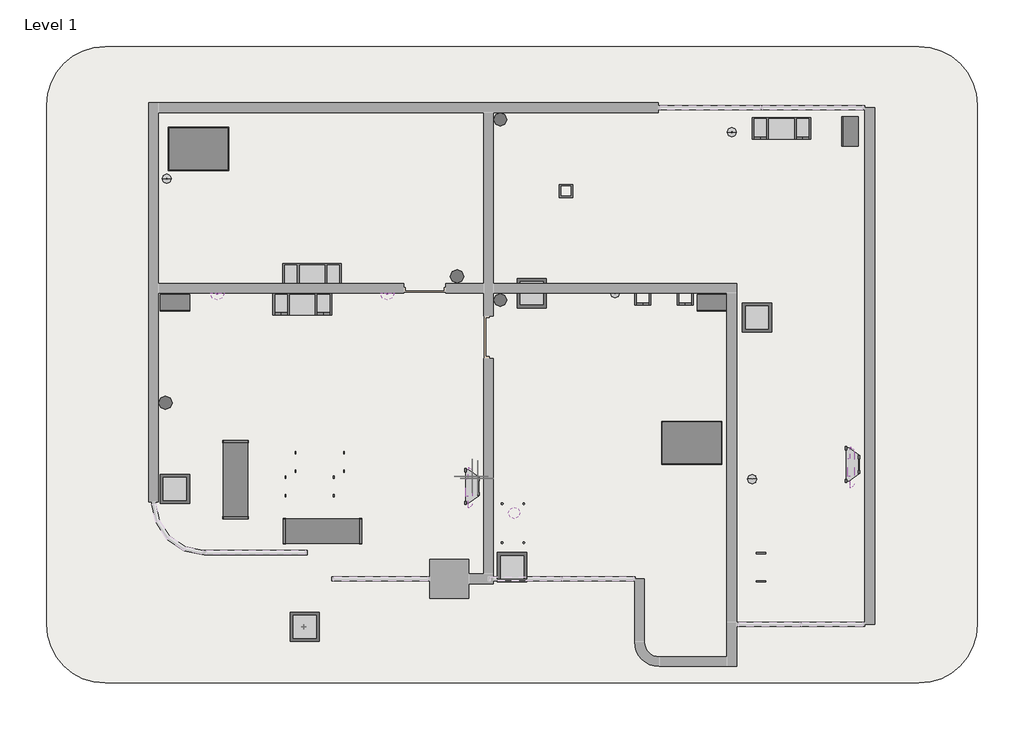
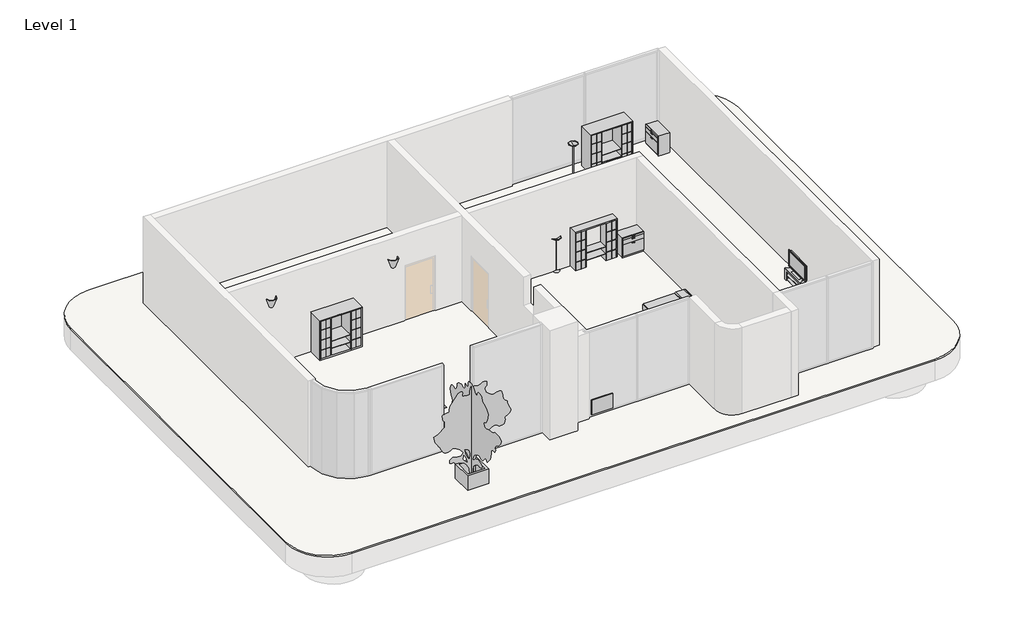
# One storey, part 2 of 2: 72 furniture elements, 8 geographic elements, 7 light fixtures, 4 proxies, 1 slab.
"""IFC4 building model written with IfcOpenShell, lengths in millimetres."""

from ifc_helpers import new_model, si_unit, point, frame, frame_2d, origin, place, context, project, spatial, polyline, circle_curve, trimmed, segment, composite_curve, outline, extrude, transform, mapped, element, save
from components import recycle_bin_round_recycle_bin_round_6e7ed866, furniture_c8abb964, furniture_cf0b6580, furniture_1a2ca15e, furniture_e1dba61b, furniture_56245f3a, furniture_fdf74506, tv_stand_tv_stand_6ce107e5, furniture_92191dda, furniture_2c34a4f9, furniture_905aceb5, furniture_027a2ad9, geographic_element_4c884dac, rpc_shrub_9ef344a8, rpc_tree_deciduous_japanese_cherry_15_e499737d, light_fixture_120v_8a54b260, sconce_light_uplight_100w_277v_9e84f6ed, table_lamp_standard_100w_120v_6e8cd8b1

model = new_model("IFC4")

# Units and contexts
model_context = context("Model", 3, world=origin())
ifc_project = project(units=[si_unit("LENGTHUNIT", "METRE", prefix="MILLI")], contexts=[model_context])

# Site, building, storey
site = spatial("IfcSite", under=ifc_project)
building = spatial("IfcBuilding", under=site)
storey = spatial("IfcBuildingStorey", under=building, Name="Level 1", Elevation=0.0)

# Proxies
placement = place(None, origin())
recycle_bin_round_recycle_bin_round_shape = recycle_bin_round_recycle_bin_round_6e7ed866(model_context)
element("IfcBuildingElementProxy", 1, Name="Recycle Bin-Round : Recycle Bin-Round", ObjectType="Recycle Bin-Round : Recycle Bin-Round", at=placement, inside=storey, context=model_context, shape_type="MappedRepresentation", body=[
    mapped(recycle_bin_round_recycle_bin_round_shape, transform((-16356.1155088, 1608.9091958, 990.6), x_axis=(1.0, 0.0, 0.0), y_axis=(0.0, 1.0, 0.0), z_axis=(0.0, 0.0, 1.0))),
])
element("IfcBuildingElementProxy", 2, Name="Recycle Bin-Round : Recycle Bin-Round", ObjectType="Recycle Bin-Round : Recycle Bin-Round", at=placement, inside=storey, context=model_context, shape_type="MappedRepresentation", body=[
    mapped(recycle_bin_round_recycle_bin_round_shape, transform((-5939.736879, 10427.3437739, 990.6), x_axis=(1.0, 0.0, 0.0), y_axis=(0.0, 1.0, 0.0), z_axis=(0.0, 0.0, 1.0))),
])
element("IfcBuildingElementProxy", 3, Name="Recycle Bin-Round : Recycle Bin-Round", ObjectType="Recycle Bin-Round : Recycle Bin-Round", at=placement, inside=storey, context=model_context, shape_type="MappedRepresentation", body=[
    mapped(recycle_bin_round_recycle_bin_round_shape, transform((-5939.736879, 4809.3091958, 990.6), x_axis=(1.0, 0.0, 0.0), y_axis=(0.0, 1.0, 0.0), z_axis=(0.0, 0.0, 1.0))),
])
element("IfcBuildingElementProxy", 4, Name="Recycle Bin-Round : Recycle Bin-Round", ObjectType="Recycle Bin-Round : Recycle Bin-Round", at=placement, inside=storey, context=model_context, shape_type="MappedRepresentation", body=[
    mapped(recycle_bin_round_recycle_bin_round_shape, transform((-7285.936879, 5545.9091958, 990.6), x_axis=(1.0, 0.0, 0.0), y_axis=(0.0, 1.0, 0.0), z_axis=(0.0, 0.0, 1.0))),
])

# Furniture
furniture_shape = furniture_c8abb964(model_context)
element("IfcFurniture", 5, ObjectType="Bed-Box : Double 53\" x 74\"", at=placement, inside=storey, context=model_context, shape_type="MappedRepresentation", body=[
    mapped(furniture_shape, transform((-15561.845017, 9173.7913149, 990.6), x_axis=(0.0, 1.0000000000000002, 0.0), y_axis=(-1.0000000000000002, 0.0, 0.0), z_axis=(0.0, 0.0, 1.0))),
])
element("IfcFurniture", 6, ObjectType="Bed-Box : Double 53\" x 74\"", at=placement, inside=storey, context=model_context, shape_type="MappedRepresentation", body=[
    mapped(furniture_shape, transform((250.9926292, 703.4616548, 990.6), x_axis=(0.0, -1.0000000000000004, 0.0), y_axis=(1.0000000000000004, 0.0, 0.0), z_axis=(0.0, 0.0, 1.0))),
])
furniture_2_shape = furniture_cf0b6580(model_context)
element("IfcFurniture", 7, ObjectType="Entertainment Center : 72\" x 72\" x 24\"", at=placement, inside=storey, context=model_context, shape_type="MappedRepresentation", body=[
    mapped(furniture_2_shape, transform((2806.4150045, 10592.4437739, 990.6), x_axis=(1.0000000000000002, 0.0, 0.0), y_axis=(0.0, 1.0000000000000002, 0.0), z_axis=(0.0, 0.0, 1.0))),
])
element("IfcFurniture", 8, ObjectType="Entertainment Center : 72\" x 72\" x 24\"", at=placement, inside=storey, context=model_context, shape_type="MappedRepresentation", body=[
    mapped(furniture_2_shape, transform((-847.036879, 5431.6091958, 914.4), x_axis=(1.0, 0.0, 0.0), y_axis=(0.0, 1.0, 0.0), z_axis=(0.0, 0.0, 1.0))),
])
element("IfcFurniture", 9, ObjectType="Entertainment Center : 72\" x 72\" x 24\"", at=placement, inside=storey, context=model_context, shape_type="MappedRepresentation", body=[
    mapped(furniture_2_shape, transform((-11794.436879, 6041.2091958, 990.6), x_axis=(1.0, 0.0, 0.0), y_axis=(0.0, 1.0, 0.0), z_axis=(0.0, 0.0, 1.0))),
])
element("IfcFurniture", 10, ObjectType="Entertainment Center : 72\" x 72\" x 24\"", at=placement, inside=storey, context=model_context, shape_type="MappedRepresentation", body=[
    mapped(furniture_2_shape, transform((-12099.236879, 5126.8091958, 990.6), x_axis=(1.0, 0.0, 0.0), y_axis=(0.0, 1.0, 0.0), z_axis=(0.0, 0.0, 1.0))),
])
furniture_3_shape = furniture_1a2ca15e(model_context)
element("IfcFurniture", 11, ObjectType="Sofa-Pensi : 84\"", at=placement, inside=storey, context=model_context, shape_type="MappedRepresentation", body=[
    mapped(furniture_3_shape, transform((-13881.9056728, -1065.3624761, 990.6), x_axis=(0.0, 1.0000000000000002, 0.0), y_axis=(-1.0000000000000002, 0.0, 0.0), z_axis=(0.0, 0.0, 1.0))),
])
element("IfcFurniture", 12, ObjectType="Sofa-Pensi : 84\"", at=placement, inside=storey, context=model_context, shape_type="MappedRepresentation", body=[
    mapped(furniture_3_shape, transform((-11188.0092588, -2089.0809681, 990.6), x_axis=(-1.0000000000000004, 0.0, 0.0), y_axis=(0.0, -1.0000000000000004, 0.0), z_axis=(0.0, 0.0, 1.0))),
])
furniture_4_shape = furniture_e1dba61b(model_context)
element("IfcFurniture", 13, ObjectType="Storage Pedestal : 20\" x 36\" x 36\"", at=placement, inside=storey, context=model_context, shape_type="MappedRepresentation", body=[
    mapped(furniture_4_shape, transform((-15881.614365, 5654.7275719, 990.6), x_axis=(1.0, 0.0, 0.0), y_axis=(0.0, 1.0, 0.0), z_axis=(0.0, 0.0, 1.0))),
])
element("IfcFurniture", 14, ObjectType="Storage Pedestal : 20\" x 36\" x 36\"", at=placement, inside=storey, context=model_context, shape_type="MappedRepresentation", body=[
    mapped(furniture_4_shape, transform((831.585635, 5654.7275719, 990.6), x_axis=(1.0, 0.0, 0.0), y_axis=(0.0, 1.0, 0.0), z_axis=(0.0, 0.0, 1.0))),
])
element("IfcFurniture", 15, ObjectType="Storage Pedestal : 20\" x 36\" x 36\"", at=placement, inside=storey, context=model_context, shape_type="MappedRepresentation", body=[
    mapped(furniture_4_shape, transform((5874.3333806, 9874.3866819, 990.6), x_axis=(0.0, -1.0000000000000004, 0.0), y_axis=(1.0000000000000004, 0.0, 0.0), z_axis=(0.0, 0.0, 1.0))),
])
furniture_5_shape = furniture_56245f3a(model_context)
element("IfcFurniture", 16, ObjectType="TV - Flat Screen : 32\"", at=placement, inside=storey, context=model_context, shape_type="MappedRepresentation", body=[
    mapped(furniture_5_shape, transform((-6719.9192755, 207.788288, 0.0), x_axis=(0.0, 1.0000000000000002, 0.0), y_axis=(-1.0000000000000002, 0.0, 0.0), z_axis=(0.0, 0.0, 1.0))),
])
element("IfcFurniture", 17, ObjectType="TV - Flat Screen : 32\"", at=placement, inside=storey, context=model_context, shape_type="MappedRepresentation", body=[
    mapped(furniture_5_shape, transform((-6747.2854735, 156.988288, 0.0), x_axis=(0.0, 1.0000000000000002, 0.0), y_axis=(-1.0000000000000002, 0.0, 0.0), z_axis=(0.0, 0.0, 1.0))),
])
element("IfcFurniture", 18, ObjectType="TV - Flat Screen : 32\"", at=placement, inside=storey, context=model_context, shape_type="MappedRepresentation", body=[
    mapped(furniture_5_shape, transform((-6744.9839371, 182.388288, 0.0), x_axis=(0.0, 1.0000000000000002, 0.0), y_axis=(-1.0000000000000002, 0.0, 0.0), z_axis=(0.0, 0.0, 1.0))),
])
element("IfcFurniture", 19, ObjectType="TV - Flat Screen : 32\"", at=placement, inside=storey, context=model_context, shape_type="MappedRepresentation", body=[
    mapped(furniture_5_shape, transform((-7116.5872148, -609.64629, 0.0), x_axis=(0.0, 1.0000000000000002, 0.0), y_axis=(-1.0000000000000002, 0.0, 0.0), z_axis=(0.0, 0.0, 1.0))),
])
element("IfcFurniture", 20, ObjectType="TV - Flat Screen : 32\"", at=placement, inside=storey, context=model_context, shape_type="MappedRepresentation", body=[
    mapped(furniture_5_shape, transform((-6882.2768852, 172.3357896, 0.0), x_axis=(0.0, 1.0000000000000002, 0.0), y_axis=(-1.0000000000000002, 0.0, 0.0), z_axis=(0.0, 0.0, 1.0))),
])
element("IfcFurniture", 21, ObjectType="TV - Flat Screen : 32\"", at=placement, inside=storey, context=model_context, shape_type="MappedRepresentation", body=[
    mapped(furniture_5_shape, transform((-6747.9472673, 156.988288, 0.0), x_axis=(0.0, 1.0000000000000002, 0.0), y_axis=(-1.0000000000000002, 0.0, 0.0), z_axis=(0.0, 0.0, 1.0))),
])
element("IfcFurniture", 22, ObjectType="TV - Flat Screen : 32\"", at=placement, inside=storey, context=model_context, shape_type="MappedRepresentation", body=[
    mapped(furniture_5_shape, transform((-6734.0131954, 126.95371, 0.0), x_axis=(0.0, 1.0000000000000002, 0.0), y_axis=(-1.0000000000000002, 0.0, 0.0), z_axis=(0.0, 0.0, 1.0))),
])
element("IfcFurniture", 23, ObjectType="TV - Flat Screen : 32\"", at=placement, inside=storey, context=model_context, shape_type="MappedRepresentation", body=[
    mapped(furniture_5_shape, transform((-6797.5564969, 76.15371, 0.0), x_axis=(0.0, 1.0000000000000002, 0.0), y_axis=(-1.0000000000000002, 0.0, 0.0), z_axis=(0.0, 0.0, 1.0))),
])
element("IfcFurniture", 24, ObjectType="TV - Flat Screen : 32\"", at=placement, inside=storey, context=model_context, shape_type="MappedRepresentation", body=[
    mapped(furniture_5_shape, transform((-6791.2021667, 101.55371, 0.0), x_axis=(0.0, 1.0000000000000002, 0.0), y_axis=(-1.0000000000000002, 0.0, 0.0), z_axis=(0.0, 0.0, 1.0))),
])
element("IfcFurniture", 25, ObjectType="TV - Flat Screen : 32\"", at=placement, inside=storey, context=model_context, shape_type="MappedRepresentation", body=[
    mapped(furniture_5_shape, transform((-6784.8478366, 101.55371, 0.0), x_axis=(0.0, 1.0000000000000002, 0.0), y_axis=(-1.0000000000000002, 0.0, 0.0), z_axis=(0.0, 0.0, 1.0))),
])
element("IfcFurniture", 26, ObjectType="TV - Flat Screen : 32\"", at=placement, inside=storey, context=model_context, shape_type="MappedRepresentation", body=[
    mapped(furniture_5_shape, transform((-5298.5159462, 1625.55371, 0.0), x_axis=(0.0, 1.0000000000000002, 0.0), y_axis=(-1.0000000000000002, 0.0, 0.0), z_axis=(0.0, 0.0, 1.0))),
])
element("IfcFurniture", 27, ObjectType="TV - Flat Screen : 32\"", at=placement, inside=storey, context=model_context, shape_type="MappedRepresentation", body=[
    mapped(furniture_5_shape, transform((-5407.1719896, 1574.75371, 0.0), x_axis=(0.0, 1.0000000000000002, 0.0), y_axis=(-1.0000000000000002, 0.0, 0.0), z_axis=(0.0, 0.0, 1.0))),
])
element("IfcFurniture", 28, ObjectType="TV - Flat Screen : 32\"", at=placement, inside=storey, context=model_context, shape_type="MappedRepresentation", body=[
    mapped(furniture_5_shape, transform((-5393.8163297, 1655.588288, 0.0), x_axis=(0.0, 1.0000000000000002, 0.0), y_axis=(-1.0000000000000002, 0.0, 0.0), z_axis=(0.0, 0.0, 1.0))),
])
element("IfcFurniture", 29, ObjectType="TV - Flat Screen : 32\"", at=placement, inside=storey, context=model_context, shape_type="MappedRepresentation", body=[
    mapped(furniture_5_shape, transform((-6717.1119705, 169.8646817, 0.0), x_axis=(0.0, -1.0000000000000002, 0.0), y_axis=(1.0000000000000002, 0.0, 0.0), z_axis=(0.0, 0.0, 1.0))),
])
element("IfcFurniture", 30, ObjectType="TV - Flat Screen : 32\"", at=placement, inside=storey, context=model_context, shape_type="MappedRepresentation", body=[
    mapped(furniture_5_shape, transform((-6719.8264069, 169.8646817, 0.0), x_axis=(0.0, -1.0, 0.0), y_axis=(1.0, 0.0, 0.0), z_axis=(0.0, 0.0, 1.0))),
])
furniture_6_shape = furniture_fdf74506(model_context)
element("IfcFurniture", 31, ObjectType="TV - Flat Screen : 50\"", at=placement, inside=storey, context=model_context, shape_type="MappedRepresentation", body=[
    mapped(furniture_6_shape, transform((-6792.5864683, -947.7353183, 0.0), x_axis=(0.0, -1.0, 0.0), y_axis=(1.0, 0.0, 0.0), z_axis=(0.0, 0.0, 1.0))),
])
element("IfcFurniture", 32, ObjectType="TV - Flat Screen : 50\"", at=placement, inside=storey, context=model_context, shape_type="MappedRepresentation", body=[
    mapped(furniture_6_shape, transform((-6773.7504988, -947.7353183, 0.0), x_axis=(0.0, -1.0, 0.0), y_axis=(1.0, 0.0, 0.0), z_axis=(0.0, 0.0, 1.0))),
])
element("IfcFurniture", 33, ObjectType="TV - Flat Screen : 50\"", at=placement, inside=storey, context=model_context, shape_type="MappedRepresentation", body=[
    mapped(furniture_6_shape, transform((-6675.9755026, -1031.0353183, 0.0), x_axis=(0.0, -1.0, 0.0), y_axis=(1.0, 0.0, 0.0), z_axis=(0.0, 0.0, 1.0))),
])
element("IfcFurniture", 34, ObjectType="TV - Flat Screen : 50\"", at=placement, inside=storey, context=model_context, shape_type="MappedRepresentation", body=[
    mapped(furniture_6_shape, transform((-6645.9755026, -1100.1353183, 0.0), x_axis=(0.0, -1.0, 0.0), y_axis=(1.0, 0.0, 0.0), z_axis=(0.0, 0.0, 1.0))),
])
element("IfcFurniture", 35, ObjectType="TV - Flat Screen : 50\"", at=placement, inside=storey, context=model_context, shape_type="MappedRepresentation", body=[
    mapped(furniture_6_shape, transform((5016.5763808, -407.0532386, 1498.6), x_axis=(0.0, -1.0, 0.0), y_axis=(1.0, 0.0, 0.0), z_axis=(0.0, 0.0, 1.0))),
])
element("IfcFurniture", 36, ObjectType="TV - Flat Screen : 50\"", at=placement, inside=storey, context=model_context, shape_type="MappedRepresentation", body=[
    mapped(furniture_6_shape, transform((-6665.9755026, -966.0532386, 0.0), x_axis=(0.0, -1.0, 0.0), y_axis=(1.0, 0.0, 0.0), z_axis=(0.0, 0.0, 1.0))),
])
element("IfcFurniture", 37, ObjectType="TV - Flat Screen : 50\"", at=placement, inside=storey, context=model_context, shape_type="MappedRepresentation", body=[
    mapped(furniture_6_shape, transform((-6675.9755026, -978.5532386, 0.0), x_axis=(0.0, -1.0, 0.0), y_axis=(1.0, 0.0, 0.0), z_axis=(0.0, 0.0, 1.0))),
])
element("IfcFurniture", 38, ObjectType="TV - Flat Screen : 50\"", at=placement, inside=storey, context=model_context, shape_type="MappedRepresentation", body=[
    mapped(furniture_6_shape, transform((-7108.6644621, -1050.5156256, 0.0), x_axis=(0.0, -1.0, 0.0), y_axis=(1.0, 0.0, 0.0), z_axis=(0.0, 0.0, 1.0))),
])
element("IfcFurniture", 39, ObjectType="TV - Flat Screen : 50\"", at=placement, inside=storey, context=model_context, shape_type="MappedRepresentation", body=[
    mapped(furniture_6_shape, transform((-7053.1755026, -998.5353183, 0.0), x_axis=(0.0, -1.0, 0.0), y_axis=(1.0, 0.0, 0.0), z_axis=(0.0, 0.0, 1.0))),
])
element("IfcFurniture", 40, ObjectType="TV - Flat Screen : 50\"", at=placement, inside=storey, context=model_context, shape_type="MappedRepresentation", body=[
    mapped(furniture_6_shape, transform((-6907.8179606, -1074.7353183, 0.0), x_axis=(0.0, -1.0, 0.0), y_axis=(1.0, 0.0, 0.0), z_axis=(0.0, 0.0, 1.0))),
])
element("IfcFurniture", 41, ObjectType="TV - Flat Screen : 50\"", at=placement, inside=storey, context=model_context, shape_type="MappedRepresentation", body=[
    mapped(furniture_6_shape, transform((-6796.3533592, -1049.3353183, 0.0), x_axis=(0.0, -1.0, 0.0), y_axis=(1.0, 0.0, 0.0), z_axis=(0.0, 0.0, 1.0))),
])
element("IfcFurniture", 42, ObjectType="TV - Flat Screen : 50\"", at=placement, inside=storey, context=model_context, shape_type="MappedRepresentation", body=[
    mapped(furniture_6_shape, transform((-6866.1755026, -1037.9080781, 1600.2), x_axis=(0.0, -1.0, 0.0), y_axis=(1.0, 0.0, 0.0), z_axis=(0.0, 0.0, 1.0))),
])
tv_stand_tv_stand_shape = tv_stand_tv_stand_6ce107e5(model_context)
element("IfcFurniture", 43, ObjectType="TV Stand : TV Stand", at=placement, inside=storey, context=model_context, shape_type="MappedRepresentation", body=[
    mapped(tv_stand_tv_stand_shape, transform((-6460.436879, -336.0028021, 0.0), x_axis=(0.0, -1.0, 0.0), y_axis=(1.0, 0.0, 0.0), z_axis=(0.0, 0.0, 1.0))),
])
element("IfcFurniture", 44, ObjectType="TV Stand : TV Stand", at=placement, inside=storey, context=model_context, shape_type="MappedRepresentation", body=[
    mapped(tv_stand_tv_stand_shape, transform((-6562.036879, -310.6028021, 0.0), x_axis=(0.0, -1.0, 0.0), y_axis=(1.0, 0.0, 0.0), z_axis=(0.0, 0.0, 1.0))),
])
element("IfcFurniture", 45, ObjectType="TV Stand : TV Stand", at=placement, inside=storey, context=model_context, shape_type="MappedRepresentation", body=[
    mapped(tv_stand_tv_stand_shape, transform((5244.8150045, -183.6028021, 990.6), x_axis=(0.0, -1.0, 0.0), y_axis=(1.0, 0.0, 0.0), z_axis=(0.0, 0.0, 1.0))),
])
element("IfcFurniture", 46, ObjectType="TV Stand : TV Stand", at=placement, inside=storey, context=model_context, shape_type="MappedRepresentation", body=[
    mapped(tv_stand_tv_stand_shape, transform((-6612.836879, -336.0028021, 0.0), x_axis=(0.0, -1.0, 0.0), y_axis=(1.0, 0.0, 0.0), z_axis=(0.0, 0.0, 1.0))),
])
element("IfcFurniture", 47, ObjectType="TV Stand : TV Stand", at=placement, inside=storey, context=model_context, shape_type="MappedRepresentation", body=[
    mapped(tv_stand_tv_stand_shape, transform((-6612.836879, 273.5971979, 0.0), x_axis=(0.0, -1.0, 0.0), y_axis=(1.0, 0.0, 0.0), z_axis=(0.0, 0.0, 1.0))),
])
element("IfcFurniture", 48, ObjectType="TV Stand : TV Stand", at=placement, inside=storey, context=model_context, shape_type="MappedRepresentation", body=[
    mapped(tv_stand_tv_stand_shape, transform((-6612.836879, 1340.3971979, 0.0), x_axis=(0.0, -1.0, 0.0), y_axis=(1.0, 0.0, 0.0), z_axis=(0.0, 0.0, 1.0))),
])
element("IfcFurniture", 49, ObjectType="TV Stand : TV Stand", at=placement, inside=storey, context=model_context, shape_type="MappedRepresentation", body=[
    mapped(tv_stand_tv_stand_shape, transform((-6562.036879, -1123.4028021, 0.0), x_axis=(0.0, -1.0, 0.0), y_axis=(1.0, 0.0, 0.0), z_axis=(0.0, 0.0, 1.0))),
])
element("IfcFurniture", 50, ObjectType="TV Stand : TV Stand", at=placement, inside=storey, context=model_context, shape_type="MappedRepresentation", body=[
    mapped(tv_stand_tv_stand_shape, transform((-6460.436879, -1098.0028021, 0.0), x_axis=(0.0, -1.0, 0.0), y_axis=(1.0, 0.0, 0.0), z_axis=(0.0, 0.0, 1.0))),
])
element("IfcFurniture", 51, ObjectType="TV Stand : TV Stand", at=placement, inside=storey, context=model_context, shape_type="MappedRepresentation", body=[
    mapped(tv_stand_tv_stand_shape, transform((-6587.436879, -869.4028021, 990.6), x_axis=(0.0, -1.0000000000000004, 0.0), y_axis=(1.0000000000000004, 0.0, 0.0), z_axis=(0.0, 0.0, 1.0))),
])
furniture_7_shape = furniture_92191dda(model_context)
element("IfcFurniture", 52, ObjectType="Table-Dining : 30\" x 84\" x 22\"", at=placement, inside=storey, context=model_context, shape_type="MappedRepresentation", body=[
    mapped(furniture_7_shape, transform((-12819.204431, -195.4219928, 0.0), x_axis=(0.0, 1.0000000000000002, 0.0), y_axis=(-1.0000000000000002, 0.0, 0.0), z_axis=(0.0, 0.0, 1.0))),
])
element("IfcFurniture", 53, ObjectType="Table-Dining : 30\" x 84\" x 22\"", at=placement, inside=storey, context=model_context, shape_type="MappedRepresentation", body=[
    mapped(furniture_7_shape, transform((-12286.5497421, -518.3797264, 0.0), x_axis=(-1.0000000000000004, 0.0, 0.0), y_axis=(0.0, -1.0000000000000004, 0.0), z_axis=(0.0, 0.0, 1.0))),
])
element("IfcFurniture", 54, ObjectType="Table-Dining : 30\" x 84\" x 22\"", at=placement, inside=storey, context=model_context, shape_type="MappedRepresentation", body=[
    mapped(furniture_7_shape, transform((-12286.5497421, -365.9797264, 0.0), x_axis=(-1.0, 0.0, 0.0), y_axis=(0.0, -1.0, 0.0), z_axis=(0.0, 0.0, 1.0))),
])
element("IfcFurniture", 55, ObjectType="Table-Dining : 30\" x 84\" x 22\"", at=placement, inside=storey, context=model_context, shape_type="MappedRepresentation", body=[
    mapped(furniture_7_shape, transform((-12438.9497421, -518.3797264, 0.0), x_axis=(-1.0, 0.0, 0.0), y_axis=(0.0, -1.0, 0.0), z_axis=(0.0, 0.0, 1.0))),
])
element("IfcFurniture", 56, ObjectType="Table-Dining : 30\" x 84\" x 22\"", at=placement, inside=storey, context=model_context, shape_type="MappedRepresentation", body=[
    mapped(furniture_7_shape, transform((-12480.5652404, -542.4184009, 0.0), x_axis=(-1.0, 0.0, 0.0), y_axis=(0.0, -1.0, 0.0), z_axis=(0.0, 0.0, 1.0))),
])
element("IfcFurniture", 57, ObjectType="Table-Dining : 30\" x 84\" x 22\"", at=placement, inside=storey, context=model_context, shape_type="MappedRepresentation", body=[
    mapped(furniture_7_shape, transform((-11854.7497421, -899.3797264, 990.6), x_axis=(-1.0, 0.0, 0.0), y_axis=(0.0, -1.0, 0.0), z_axis=(0.0, 0.0, 1.0))),
])
element("IfcFurniture", 58, ObjectType="Table-Dining : 30\" x 84\" x 22\"", at=placement, inside=storey, context=model_context, shape_type="MappedRepresentation", body=[
    mapped(furniture_7_shape, transform((-12743.7497421, 91.2202736, 0.0), x_axis=(-1.0, 0.0, 0.0), y_axis=(0.0, -1.0, 0.0), z_axis=(0.0, 0.0, 1.0))),
])
element("IfcFurniture", 59, ObjectType="Table-Dining : 30\" x 84\" x 22\"", at=placement, inside=storey, context=model_context, shape_type="MappedRepresentation", body=[
    mapped(furniture_7_shape, transform((-12743.7497421, 396.0202736, 0.0), x_axis=(-1.0, 0.0, 0.0), y_axis=(0.0, -1.0, 0.0), z_axis=(0.0, 0.0, 1.0))),
])
element("IfcFurniture", 60, ObjectType="Table-Dining : 30\" x 84\" x 22\"", at=placement, inside=storey, context=model_context, shape_type="MappedRepresentation", body=[
    mapped(furniture_7_shape, transform((-12705.5342656, 301.8094291, 0.0), x_axis=(-1.0, 0.0, 0.0), y_axis=(0.0, -1.0, 0.0), z_axis=(0.0, 0.0, 1.0))),
])
element("IfcFurniture", 61, ObjectType="Table-Dining : 30\" x 84\" x 22\"", at=placement, inside=storey, context=model_context, shape_type="MappedRepresentation", body=[
    mapped(furniture_7_shape, transform((-12702.2664799, 298.5416433, 0.0), x_axis=(-1.0, 0.0, 0.0), y_axis=(0.0, -1.0, 0.0), z_axis=(0.0, 0.0, 1.0))),
])
element("IfcFurniture", 62, ObjectType="Table-Dining : 30\" x 84\" x 22\"", at=placement, inside=storey, context=model_context, shape_type="MappedRepresentation", body=[
    mapped(furniture_7_shape, transform((-12758.6691759, 225.6045363, 0.0), x_axis=(-1.0, 0.0, 0.0), y_axis=(0.0, -1.0, 0.0), z_axis=(0.0, 0.0, 1.0))),
])
element("IfcFurniture", 63, ObjectType="Table-Dining : 30\" x 84\" x 22\"", at=placement, inside=storey, context=model_context, shape_type="MappedRepresentation", body=[
    mapped(furniture_7_shape, transform((-12593.5140516, 599.3766596, 0.0), x_axis=(-1.0, 0.0, 0.0), y_axis=(0.0, -1.0, 0.0), z_axis=(0.0, 0.0, 1.0))),
])
element("IfcFurniture", 64, ObjectType="Table-Dining : 30\" x 84\" x 22\"", at=placement, inside=storey, context=model_context, shape_type="MappedRepresentation", body=[
    mapped(furniture_7_shape, transform((-11054.963684, 460.2986602, 0.0), x_axis=(-1.0, 0.0, 0.0), y_axis=(0.0, -1.0, 0.0), z_axis=(0.0, 0.0, 1.0))),
])
element("IfcFurniture", 65, ObjectType="Table-Dining : 30\" x 84\" x 22\"", at=placement, inside=storey, context=model_context, shape_type="MappedRepresentation", body=[
    mapped(furniture_7_shape, transform((-10420.420312, 8.2951624, 0.0), x_axis=(-1.0, 0.0, 0.0), y_axis=(0.0, -1.0, 0.0), z_axis=(0.0, 0.0, 1.0))),
])
element("IfcFurniture", 66, ObjectType="Table-Dining : 30\" x 84\" x 22\"", at=placement, inside=storey, context=model_context, shape_type="MappedRepresentation", body=[
    mapped(furniture_7_shape, transform((-10272.6499377, -322.0150861, 0.0), x_axis=(-1.0, 0.0, 0.0), y_axis=(0.0, -1.0, 0.0), z_axis=(0.0, 0.0, 1.0))),
])
element("IfcFurniture", 67, ObjectType="Table-Dining : 30\" x 84\" x 22\"", at=placement, inside=storey, context=model_context, shape_type="MappedRepresentation", body=[
    mapped(furniture_7_shape, transform((-10941.9628095, 860.1479083, 0.0), x_axis=(-1.0, 0.0, 0.0), y_axis=(0.0, -1.0, 0.0), z_axis=(0.0, 0.0, 1.0))),
])
element("IfcFurniture", 68, ObjectType="Table-Dining : 30\" x 84\" x 22\"", at=placement, inside=storey, context=model_context, shape_type="MappedRepresentation", body=[
    mapped(furniture_7_shape, transform((-12196.3528819, -327.801882, 0.0), x_axis=(1.0, 0.0, 0.0), y_axis=(0.0, 1.0, 0.0), z_axis=(0.0, 0.0, 1.0))),
])
element("IfcFurniture", 69, ObjectType="Table-Dining : 30\" x 84\" x 22\"", at=placement, inside=storey, context=model_context, shape_type="MappedRepresentation", body=[
    mapped(furniture_7_shape, transform((-12275.6729765, -531.001882, 0.0), x_axis=(1.0, 0.0, 0.0), y_axis=(0.0, 1.0, 0.0), z_axis=(0.0, 0.0, 1.0))),
])
element("IfcFurniture", 70, ObjectType="Table-Dining : 30\" x 84\" x 22\"", at=placement, inside=storey, context=model_context, shape_type="MappedRepresentation", body=[
    mapped(furniture_7_shape, transform((-12117.5026456, 184.8326961, 0.0), x_axis=(1.0, 0.0, 0.0), y_axis=(0.0, 1.0, 0.0), z_axis=(0.0, 0.0, 1.0))),
])
element("IfcFurniture", 71, ObjectType="Table-Dining : 30\" x 84\" x 22\"", at=placement, inside=storey, context=model_context, shape_type="MappedRepresentation", body=[
    mapped(furniture_7_shape, transform((-11965.1026456, 184.8326961, 0.0), x_axis=(1.0, 0.0, 0.0), y_axis=(0.0, 1.0, 0.0), z_axis=(0.0, 0.0, 1.0))),
])
element("IfcFurniture", 72, ObjectType="Table-Dining : 30\" x 84\" x 22\"", at=placement, inside=storey, context=model_context, shape_type="MappedRepresentation", body=[
    mapped(furniture_7_shape, transform((-12422.3026456, 2928.0326961, 0.0), x_axis=(1.0, 0.0, 0.0), y_axis=(0.0, 1.0, 0.0), z_axis=(0.0, 0.0, 1.0))),
])
element("IfcFurniture", 73, ObjectType="Table-Dining : 30\" x 84\" x 22\"", at=placement, inside=storey, context=model_context, shape_type="MappedRepresentation", body=[
    mapped(furniture_7_shape, transform((-11577.7526456, -323.1673039, 990.6), x_axis=(1.0, 0.0, 0.0), y_axis=(0.0, 1.0, 0.0), z_axis=(0.0, 0.0, 1.0))),
])
furniture_8_shape = furniture_2c34a4f9(model_context)
element("IfcFurniture", 74, ObjectType="Table-Dining Oval : 36\" x 72\"", at=placement, inside=storey, context=model_context, shape_type="MappedRepresentation", body=[
    mapped(furniture_8_shape, transform((-5904.1352396, -1735.7711321, 990.6), x_axis=(0.0, 1.0000000000000002, 0.0), y_axis=(-1.0000000000000002, 0.0, 0.0), z_axis=(0.0, 0.0, 1.0))),
])
furniture_9_shape = furniture_905aceb5(model_context)
element("IfcFurniture", 75, ObjectType="Table-Dining Round w Chairs : 36\" Diameter", at=placement, inside=storey, context=model_context, shape_type="MappedRepresentation", body=[
    mapped(furniture_9_shape, transform((-3998.7188462, 8389.7224624, 990.6), x_axis=(1.0, 0.0, 0.0), y_axis=(0.0, 1.0, 0.0), z_axis=(0.0, 0.0, 1.0))),
])
furniture_10_shape = furniture_027a2ad9(model_context)
element("IfcFurniture", 76, ObjectType="Table-Ellipse : 72\" x 36\"", at=placement, inside=storey, context=model_context, shape_type="MappedRepresentation", body=[
    mapped(furniture_10_shape, transform((2175.563121, -3509.1908042, 990.6), x_axis=(0.0, 1.0000000000000002, 0.0), y_axis=(-1.0000000000000002, 0.0, 0.0), z_axis=(0.0, 0.0, 1.0))),
])

# Geographic elements
geographic_element_shape = geographic_element_4c884dac(model_context)
element("IfcGeographicElement", 77, ObjectType="Planter : 36\" x 36\"", at=placement, inside=storey, context=model_context, shape_type="MappedRepresentation", body=[
    mapped(geographic_element_shape, transform((-5571.436879, -3509.1908042, 990.6), x_axis=(1.0, 0.0, 0.0), y_axis=(0.0, 1.0, 0.0), z_axis=(0.0, 0.0, 1.0))),
])
element("IfcGeographicElement", 78, ObjectType="Planter : 36\" x 36\"", at=placement, inside=storey, context=model_context, shape_type="MappedRepresentation", body=[
    mapped(geographic_element_shape, transform((-16061.636879, -1070.7908042, 990.6), x_axis=(1.0, 0.0, 0.0), y_axis=(0.0, 1.0, 0.0), z_axis=(0.0, 0.0, 1.0))),
])
element("IfcGeographicElement", 79, ObjectType="Planter : 36\" x 36\"", at=placement, inside=storey, context=model_context, shape_type="MappedRepresentation", body=[
    mapped(geographic_element_shape, transform((2044.4150045, 4263.2091958, 990.6), x_axis=(1.0, 0.0, 0.0), y_axis=(0.0, 1.0, 0.0), z_axis=(0.0, 0.0, 1.0))),
])
element("IfcGeographicElement", 80, ObjectType="Planter : 36\" x 36\"", at=placement, inside=storey, context=model_context, shape_type="MappedRepresentation", body=[
    mapped(geographic_element_shape, transform((-4961.836879, 5025.2091958, 990.6), x_axis=(1.0, 0.0, 0.0), y_axis=(0.0, 1.0, 0.0), z_axis=(0.0, 0.0, 1.0))),
])
element("IfcGeographicElement", 81, ObjectType="Planter : 36\" x 36\"", at=placement, inside=storey, context=model_context, shape_type="MappedRepresentation", body=[
    mapped(geographic_element_shape, transform((-12023.036879, -5363.3908042, 914.4), x_axis=(1.0, 0.0, 0.0), y_axis=(0.0, 1.0, 0.0), z_axis=(0.0, 0.0, 1.0))),
])
rpc_shrub_shape = rpc_shrub_9ef344a8(model_context)
element("IfcGeographicElement", 82, ObjectType="RPC Shrub", at=placement, inside=storey, context=model_context, shape_type="MappedRepresentation", body=[
    mapped(rpc_shrub_shape, transform((-6816.036879, -685.1562261, 0.0), x_axis=(1.0, 0.0, 0.0), y_axis=(0.0, 1.0, 0.0), z_axis=(0.0, 0.0, 1.0))),
])
element("IfcGeographicElement", 83, ObjectType="RPC Shrub", at=placement, inside=storey, context=model_context, shape_type="MappedRepresentation", body=[
    mapped(rpc_shrub_shape, transform((-6638.236879, -735.9562261, 0.0), x_axis=(1.0, 0.0, 0.0), y_axis=(0.0, 1.0, 0.0), z_axis=(0.0, 0.0, 1.0))),
])
rpc_tree_deciduous_japanese_cherry_15_shape = rpc_tree_deciduous_japanese_cherry_15_e499737d(model_context)
element("IfcGeographicElement", 84, ObjectType="RPC Tree - Deciduous : Japanese Cherry - 15'", at=placement, inside=storey, context=model_context, shape_type="MappedRepresentation", body=[
    mapped(rpc_tree_deciduous_japanese_cherry_15_shape, transform((-12048.436879, -5363.3908042, 914.4), x_axis=(1.0, 0.0, 0.0), y_axis=(0.0, 1.0, 0.0), z_axis=(0.0, 0.0, 1.0))),
])

# Light fixtures
light_fixture_120v_shape = light_fixture_120v_8a54b260(model_context)
element("IfcLightFixture", 85, ObjectType="120V", at=placement, inside=storey, context=model_context, shape_type="MappedRepresentation", body=[
    mapped(light_fixture_120v_shape, transform((1261.163121, 10033.6437739, 990.6), x_axis=(1.0, 0.0, 0.0), y_axis=(0.0, 1.0, 0.0), z_axis=(0.0, 0.0, 1.0))),
])
element("IfcLightFixture", 86, ObjectType="120V", at=placement, inside=storey, context=model_context, shape_type="MappedRepresentation", body=[
    mapped(light_fixture_120v_shape, transform((1892.0150045, -765.9908042, 990.6), x_axis=(1.0, 0.0, 0.0), y_axis=(0.0, 1.0, 0.0), z_axis=(0.0, 0.0, 1.0))),
])
element("IfcLightFixture", 87, ObjectType="120V", at=placement, inside=storey, context=model_context, shape_type="MappedRepresentation", body=[
    mapped(light_fixture_120v_shape, transform((-2371.036879, 5025.2091958, 990.6), x_axis=(1.0, 0.0, 0.0), y_axis=(0.0, 1.0, 0.0), z_axis=(0.0, 0.0, 1.0))),
])
element("IfcLightFixture", 88, ObjectType="120V", at=placement, inside=storey, context=model_context, shape_type="MappedRepresentation", body=[
    mapped(light_fixture_120v_shape, transform((-16315.636879, 8585.8437739, 990.6), x_axis=(1.0, 0.0, 0.0), y_axis=(0.0, 1.0, 0.0), z_axis=(0.0, 0.0, 1.0))),
])
sconce_light_uplight_100w_277v_shape = sconce_light_uplight_100w_277v_9e84f6ed(model_context)
element("IfcLightFixture", 89, ObjectType="Sconce Light - Uplight : 100W - 277V", at=placement, inside=storey, context=model_context, shape_type="MappedRepresentation", body=[
    mapped(sconce_light_uplight_100w_277v_shape, transform((-9457.636879, 5177.6091958, 1923.6784847), x_axis=(-1.0, 0.0, 0.0), y_axis=(0.0, -1.0, 0.0), z_axis=(0.0, 0.0, 1.0))),
])
element("IfcLightFixture", 90, ObjectType="Sconce Light - Uplight : 100W - 277V", at=placement, inside=storey, context=model_context, shape_type="MappedRepresentation", body=[
    mapped(sconce_light_uplight_100w_277v_shape, transform((-14743.2155088, 5177.6091958, 1950.9773785), x_axis=(-1.0, 0.0, 0.0), y_axis=(0.0, -1.0, 0.0), z_axis=(0.0, 0.0, 1.0))),
])
table_lamp_standard_100w_120v_shape = table_lamp_standard_100w_120v_6e8cd8b1(model_context)
element("IfcLightFixture", 91, ObjectType="Table Lamp - Standard : 60W - 120V", at=placement, inside=storey, context=model_context, shape_type="MappedRepresentation", body=[
    mapped(table_lamp_standard_100w_120v_shape, transform((-5507.936879, -1820.0908042, 1905.0), x_axis=(1.0, 0.0, 0.0), y_axis=(0.0, 1.0, 0.0), z_axis=(0.0, 0.0, 1.0))),
])

# Slab
element("IfcSlab", 92, ObjectType="Generic - 3\"", at=placement, inside=storey, context=model_context, shape_type="SweptSolid", body=[
    extrude(outline(composite_curve([segment(polyline([(-18224.7849955, 12700.6437739), (7073.6150045, 12700.6437739)]), True, "CONTINUOUS"), segment(trimmed(circle_curve(frame_2d((7073.6150045, 10871.8437739)), 1828.8), [point((7073.6150045, 12700.6437739))], [point((8902.4150045, 10871.8437739))], False, "CARTESIAN"), True, "CONTINUOUS"), segment(polyline([(8902.4150045, 10871.8437739), (8902.4150045, -5282.5562261)]), True, "CONTINUOUS"), segment(trimmed(circle_curve(frame_2d((7073.6150045, -5282.5562261)), 1828.8), [point((8902.4150045, -5282.5562261))], [point((7073.6150045, -7111.3562261))], False, "CARTESIAN"), True, "CONTINUOUS"), segment(polyline([(7073.6150045, -7111.3562261), (-18224.7849955, -7111.3562261)]), True, "CONTINUOUS"), segment(trimmed(circle_curve(frame_2d((-18224.7849955, -5282.5562261)), 1828.8), [point((-18224.7849955, -7111.3562261))], [point((-20053.5849955, -5282.5562261))], False, "CARTESIAN"), True, "CONTINUOUS"), segment(polyline([(-20053.5849955, -5282.5562261), (-20053.5849955, 10871.8437739)]), True, "CONTINUOUS"), segment(trimmed(circle_curve(frame_2d((-18224.7849955, 10871.8437739)), 1828.8), [point((-20053.5849955, 10871.8437739))], [point((-18224.7849955, 12700.6437739))], False, "CARTESIAN"), True, "CONTINUOUS")], self_intersect=False)), frame((0.0, 0.0, 914.4), z_axis=(0.0, 0.0, 1.0), x_axis=(1.0, 0.0, 0.0)), (0.0, 0.0, 1.0), 76.2),
])

save(model, "model.ifc")

# Revit data of these elements
# Type "Recycle Bin-Round : Recycle Bin-Round"
#   Default Elevation = 0
# Type "Bed-Box : Double 53\" x 74\""
#   Assembly Code = "E2020200"
#   Length = 6' - 2"
#   Width = 4' - 5"
#   Frame Material = Birch
#   Mattress Material = Linen, White
#   Default Elevation = 0
# Type "Entertainment Center : 72\" x 72\" x 24\""
#   Assembly Code = "E2020200"
#   Center Width = 2' - 8"
#   Depth = 2' - 0"
#   Height = 6' - 0"
#   Width = 6' - 0"
#   Material = none
#   Default Elevation = 0
# Type "Sofa-Pensi : 84\""
#   Assembly Code = "E2020200"
#   Length = 8' - 0"
#   Frame Material = Cherry
#   Seat Material = Linen, Beige
#   Feet Material = Steel, Chrome Plated
#   Default Elevation = 0
# Type "Storage Pedestal : 20\" x 36\" x 36\""
#   Assembly Code = "E2020"
#   Depth = 1' - 8"
#   Height = 3' - 0"
#   Width = 3' - 0"
#   Cabinet Material = Steel, Paint Finish, Ivory, Glossy
#   Handles Material = Steel, Chrome Plated
#   Default Elevation = 0
# Type "TV - Flat Screen : 32\""
#   SinAng = 0' - 0.0193"
#   L = 2' - 3.79372"
#   H = 1' - 3.6354"
#   Thickness = 0' - 4.33071"
#   Diagonal = 2' - 7.88976"
#   CosAng = 0' - 0.03431"
#   Stand [instance default] = yes
#   Default Elevation = 0
# Type "TV - Flat Screen : 50\""
#   SinAng = 0' - 0.0193"
#   L = 3' - 7.57782"
#   H = 2' - 0.51477"
#   Thickness = 0' - 4.33071"
#   Diagonal = 4' - 2"
#   CosAng = 0' - 0.03431"
#   Stand [instance default] = yes
#   Default Elevation = 0
# Type "TV Stand : TV Stand"
#   Depth = 1' - 6"
#   Width = 3' - 8"
#   Height = 1' - 7 1/2"
#   Finish = Melamine - Gray
#   Default Elevation = 0
# Type "Table-Dining : 30\" x 84\" x 22\""
#   Assembly Code = "E2020200"
#   Height = 1' - 10"
#   Length = 7' - 0"
#   Width = 2' - 6"
#   Base Material = Steel, Chrome Plated
#   Top Material = Glass - Clear, Grey
#   Default Elevation = 0
# Type "Table-Dining Oval : 36\" x 72\""
#   Assembly Code = "E2020200"
#   Length = 6' - 0"
#   Width = 3' - 0"
#   Base Material = Steel, Chrome Plated
#   Top Material = Glass - Clear, Grey
#   Default Elevation = 0
#   Description = (empty or 0)
# Type "Table-Dining Round w Chairs : 36\" Diameter"
#   Assembly Code = "E2020200"
#   Radius = 1' - 6"
#   Diameter = 3' - 0"
#   Height = 2' - 6"
#   Chairs = 4
#   Base Material = Pine
#   Top Material = Laminate, Linen, Matte
#   Default Elevation = 0
# Type "Table-Ellipse : 72\" x 36\""
#   Assembly Code = "E2020200"
#   Half Width = 1' - 6"
#   Half Length = 3' - 0"
#   Height = 2' - 6"
#   Length = 6' - 0"
#   Width = 3' - 0"
#   Base Material = Birch
#   Top Material = Laminate - Black
#   Default Elevation = 0
# Type "Planter : 36\" x 36\""
#   Depth = 3' - 0"
#   Height = 2' - 6"
#   Width = 3' - 0"
#   Material = Concrete, Precast
# Type "RPC Shrub"
#   built-in parameter 1005198 = "{2, 15},{39, RPC-16-G0FT-Q7G0-0DUH-W000-ST1L-LVER-AU},{1, 0},{1, 0},{2, 13},{1, 8},{5, Color},{1, 0},{1, 0},{3, 0.8},{3, 0.8},{3, 0.8},{1, 8},{7, BBoxMin},{1, 0},{1, 0},{1, 0},{1, 0},{1, 0},{1, 8},{7, BBoxMax},{1, 0},{1, 0},{1, 0},{1, 0},{1, 0},{2, 11},{9, RPCTypeId},{1, 0},{1, 0},{39, RPC-16-G0FT-Q7G0-0DUH-W000-ST1L-LVER-AU},{1, 6},{14, RPCPlantHeight},{1, 0},{1, 0},{1, 3},{2, 11},{7, keyword},{1, 0},{1, 0},{35, :RPCs:Shrubs [General]:Geometry:RPC},{2, 11},{8, category},{1, 0},{1, 0},{16, Shrubs [General]},{2, 11},{12, LocalizedUID},{1, 0},{1, 0},{10, Meadowlark},{2, 14},{6, Height},{1, 0},{1, 0},{1, 3},{1, 2},{16, Cast Reflections},{1, 0},{1, 0},{1, 0},{1, 2},{12, Cast Shadows},{1, 0},{1, 0},{1, 1},{1, 2},{9, Lock View},{1, 0},{1, 0},{1, 0},{1, 4},{5, ViewC},{1, 0},{1, 0},{1, 0},{21, assetlibrary_base.fbx},{1, 5},"
#   built-in parameter 1005195 = "RPC-16-G0FT-Q7G0-0DUH-W000-ST1L-LVER-AU"
#   Assembly Code = "G2050500"
#   Height = 3' - 0"
#   Default Elevation = 0
# Type "RPC Tree - Deciduous : Japanese Cherry - 15'"
#   built-in parameter 1005198 = "{2, 15},{39, RPC-16-FXGW-2MQ0-PN7K-A000-ST1L-LVER-AU},{1, 0},{1, 0},{2, 13},{1, 8},{5, Color},{1, 0},{1, 0},{3, 0.8},{3, 0.8},{3, 0.8},{1, 8},{7, BBoxMin},{1, 0},{1, 0},{1, 0},{1, 0},{1, 0},{1, 8},{7, BBoxMax},{1, 0},{1, 0},{1, 0},{1, 0},{1, 0},{2, 11},{9, RPCTypeId},{1, 0},{1, 0},{39, RPC-16-FXGW-2MQ0-PN7K-A000-ST1L-LVER-AU},{1, 6},{14, RPCPlantHeight},{1, 0},{1, 0},{2, 15},{2, 11},{7, keyword},{1, 0},{1, 0},{34, :RPCs:Trees [General]:Geometry:RPC},{2, 11},{8, category},{1, 0},{1, 0},{15, Trees [General]},{2, 11},{12, LocalizedUID},{1, 0},{1, 0},{25, Japanese Flowering Cherry},{2, 14},{6, Height},{1, 0},{1, 0},{2, 15},{1, 2},{16, Cast Reflections},{1, 0},{1, 0},{1, 0},{1, 2},{12, Cast Shadows},{1, 0},{1, 0},{1, 1},{1, 2},{9, Lock View},{1, 0},{1, 0},{1, 0},{1, 4},{5, ViewC},{1, 0},{1, 0},{1, 0},{21, assetlibrary_base.fbx},{1, 5},"
#   built-in parameter 1005195 = "RPC-16-FXGW-2MQ0-PN7K-A000-ST1L-LVER-AU"
#   Type Comments = "Japanese Cherry"
#   Assembly Code = "G2050500"
#   Height = 15' - 0"
#   Default Elevation = 0
# Type "120V"
#   Wattage Comments = "100"
#   Lamp = "T-4"
#   Assembly Code = "D5020230"
#   Wattage = 100 W
#   built-in parameter 1150110 = 1 (stored number, unit not read)
#   built-in parameter 1114217 = 1 (stored number, unit not read)
#   built-in parameter 1150109 = 1 (stored number, unit not read)
#   built-in parameter 1150113 = 1 (stored number, unit not read)
#   Lumens = 1800 lm
#   built-in parameter 1150115 = 1 (stored number, unit not read)
#   built-in parameter 1150105 = 572.958 (stored number, unit not read)
#   Light Source Symbol Size = 2' - 0"
#   built-in parameter 1150112 = 1 (stored number, unit not read)
#   built-in parameter 1150114 = 1 (stored number, unit not read)
#   built-in parameter 1150107 = 3200 (stored number, unit not read)
#   built-in parameter 1150106 = 5.72958 (stored number, unit not read)
#   Height = 5' - 0"
#   built-in parameter 1150104 = 1.67225 (stored number, unit not read)
#   Ballast Voltage = 120 V
#   built-in parameter 1114218 = 1 (stored number, unit not read)
#   built-in parameter 1150133 = 10 (stored number, unit not read)
#   Apparent Load = 100 VA
#   built-in parameter 1150134 = 3
#   built-in parameter 1150137 = 1
#   Color Filter = 16777215
#   Ballast Number of Poles = 1
#   Shade = Glass, Frosted
#   Stand = Steel, Chrome Plated
#   Dimming Lamp Color Temperature Shift = (empty or 0)
#   Default Elevation = 0
# Type "Sconce Light - Uplight : 100W - 277V"
#   Assembly Code = "D5020220"
#   Lamp = "R-30"
#   Wattage = 100 W
#   built-in parameter 1150110 = 1 (stored number, unit not read)
#   built-in parameter 1114217 = 1 (stored number, unit not read)
#   built-in parameter 1150109 = 1 (stored number, unit not read)
#   built-in parameter 1150113 = 1 (stored number, unit not read)
#   built-in parameter 1150115 = 1 (stored number, unit not read)
#   built-in parameter 1150105 = 381.972 (stored number, unit not read)
#   Light Source Symbol Size = 2' - 0"
#   built-in parameter 1150112 = 1 (stored number, unit not read)
#   built-in parameter 1150114 = 1 (stored number, unit not read)
#   built-in parameter 1150107 = 2800 (stored number, unit not read)
#   built-in parameter 1150106 = 3.81972 (stored number, unit not read)
#   built-in parameter 1150104 = 1.11484 (stored number, unit not read)
#   Ballast Voltage = 277 V
#   built-in parameter 1114218 = 1 (stored number, unit not read)
#   built-in parameter 1150133 = 10 (stored number, unit not read)
#   Lumens = 1200 lm
#   Mounting Height = 6' - 4"
#   Apparent Load = 100 VA
#   built-in parameter 1150134 = 4
#   built-in parameter 1150137 = 1
#   Color Filter = 16777215
#   built-in parameter 1140040 [instance default] = 1
#   Ballast Number of Poles = 1
#   Shade Material = Glass, Frosted
#   Dimming Lamp Color Temperature Shift = (empty or 0)
#   Default Elevation = 0
#   Wattage Comments = ""
# Type "Table Lamp - Standard : 60W - 120V"
#   Assembly Code = "D5020220"
#   Lamp = "A-19"
#   Wattage = 60 W
#   built-in parameter 1150110 = 1 (stored number, unit not read)
#   built-in parameter 1114217 = 1 (stored number, unit not read)
#   built-in parameter 1150109 = 1 (stored number, unit not read)
#   built-in parameter 1150113 = 1 (stored number, unit not read)
#   built-in parameter 1150115 = 1 (stored number, unit not read)
#   built-in parameter 1150105 = 68.0387 (stored number, unit not read)
#   Light Source Symbol Size = 2' - 0"
#   built-in parameter 1150112 = 1 (stored number, unit not read)
#   built-in parameter 1150114 = 1 (stored number, unit not read)
#   built-in parameter 1150107 = 2800 (stored number, unit not read)
#   built-in parameter 1150106 = 0.680387 (stored number, unit not read)
#   built-in parameter 1150104 = 1.32387 (stored number, unit not read)
#   Ballast Voltage = 120 V
#   built-in parameter 1114218 = 1 (stored number, unit not read)
#   built-in parameter 1150133 = 10 (stored number, unit not read)
#   Lumens = 855 lm
#   Apparent Load = 60 VA
#   built-in parameter 1150134 = 4
#   built-in parameter 1150137 = 1
#   Color Filter = 16777215
#   built-in parameter 1140040 [instance default] = 1
#   Ballast Number of Poles = 1
#   Base Material = Plastic, Opaque Black
#   Shade Material = Glass, Frosted
#   Dimming Lamp Color Temperature Shift = (empty or 0)
#   Default Elevation = 0
#   Wattage Comments = ""
# Type "Generic - 3\""
#   Assembly Code = "B1010"
#   Function = 0
#   Layers, outside or top first: 0' - 3" "Rigid insulation" (function 1)
# Elements 1, 2, 3, 4 (IfcBuildingElementProxy, "Recycle Bin-Round : Recycle Bin-Round")
#   Phase Created = New Construction
#   Materials on its faces: "Plastic - Blue", "Default - Black"
# Elements 5, 6 (IfcFurniture, "Bed-Box : Double 53\" x 74\"")
#   Phase Created = New Construction
#   Materials on its faces: "Birch", "Linen, White"
# Elements 7, 8, 9, 10 (IfcFurniture, "Entertainment Center : 72\" x 72\" x 24\"")
#   Phase Created = New Construction
#   Materials on its faces: "Steel, Chrome Plated", "Glass - Clear, Grey"
# Elements 11, 12 (IfcFurniture, "Sofa-Pensi : 84\"")
#   Phase Created = New Construction
#   Materials on its faces: "Cherry", "Linen, Beige", "Steel, Chrome Plated"
# Elements 13, 14, 15 (IfcFurniture, "Storage Pedestal : 20\" x 36\" x 36\"")
#   Phase Created = New Construction
#   Materials on its faces: "Steel, Paint Finish, Ivory, Glossy", "Steel, Chrome Plated"
# Elements 16, 17, 18, 19, 20, 21, 22, 23, 24, 25, 26, 27, 28, 29, 30 (IfcFurniture, "TV - Flat Screen : 32\"")
#   Stand = yes
#   Phase Created = New Construction
#   Materials on its faces: "TV - Black", "TV - Glass", "TV - Screen"
# Elements 31, 32, 33, 34, 35, 36, 37, 38, 39, 40, 41, 42 (IfcFurniture, "TV - Flat Screen : 50\"")
#   Stand = yes
#   Phase Created = New Construction
#   Materials on its faces: "TV - Black", "TV - Glass", "TV - Screen"
# Elements 43, 44, 45, 46, 47, 48, 49, 50, 51 (IfcFurniture, "TV Stand : TV Stand")
#   Phase Created = New Construction
#   Materials on its faces: "Melamine - Gray", "Glass - Shelves"
# Elements 52, 53, 54, 55, 56, 57, 58, 59, 60, 61, 62, 63, 64, 65, 66, 67, 68, 69, 70, 71, 72, 73 (IfcFurniture, "Table-Dining : 30\" x 84\" x 22\"")
#   Phase Created = New Construction
#   Materials on its faces: "Steel, Chrome Plated", "Glass - Clear, Grey"
# Element 74 (IfcFurniture, "Table-Dining Oval : 36\" x 72\"")
#   Phase Created = New Construction
#   Materials on its faces: "Steel, Chrome Plated", "Glass - Clear, Grey"
# Element 75 (IfcFurniture, "Table-Dining Round w Chairs : 36\" Diameter")
#   Phase Created = New Construction
#   Materials on its faces: "Pine", "Laminate, Linen, Matte"
# Element 76 (IfcFurniture, "Table-Ellipse : 72\" x 36\"")
#   Phase Created = New Construction
#   Materials on its faces: "Birch", "Laminate - Black"
# Elements 77, 78, 79, 80, 81 (IfcGeographicElement, "Planter : 36\" x 36\"")
#   Phase Created = New Construction
#   Materials on its faces: "Concrete, Precast"
# Elements 82, 83 (IfcGeographicElement, "RPC Shrub")
#   Phase Created = New Construction
# Element 84 (IfcGeographicElement, "RPC Tree - Deciduous : Japanese Cherry - 15'")
#   Phase Created = New Construction
# Element 85 (IfcLightFixture, "120V")
#   Mark = "4"
#   Phase Created = New Construction
#   Materials on its faces: "Steel, Chrome Plated", "Glass, Frosted"
# Element 86 (IfcLightFixture, "120V")
#   Mark = "5"
#   Phase Created = New Construction
#   Materials on its faces: "Steel, Chrome Plated", "Glass, Frosted"
# Element 87 (IfcLightFixture, "120V")
#   Mark = "6"
#   Phase Created = New Construction
#   Materials on its faces: "Steel, Chrome Plated", "Glass, Frosted"
# Element 88 (IfcLightFixture, "120V")
#   Mark = "7"
#   Phase Created = New Construction
#   Materials on its faces: "Steel, Chrome Plated", "Glass, Frosted"
# Element 89 (IfcLightFixture, "Sconce Light - Uplight : 100W - 277V")
#   Mark = "2"
#   built-in parameter 1140040 = 1
#   Phase Created = New Construction
#   Materials on its faces: "Glass, Frosted"
# Element 90 (IfcLightFixture, "Sconce Light - Uplight : 100W - 277V")
#   Mark = "3"
#   built-in parameter 1140040 = 1
#   Phase Created = New Construction
#   Materials on its faces: "Glass, Frosted"
# Element 91 (IfcLightFixture, "Table Lamp - Standard : 60W - 120V")
#   Mark = "1"
#   built-in parameter 1140040 = 1
#   Phase Created = New Construction
#   Materials on its faces: "Plastic, Opaque Black", "Glass, Frosted"
# Element 92 (IfcSlab, "Generic - 3\"")
#   built-in parameter 1001955 = -1.5708 (stored number, unit not read)
#   Height Offset From Level = 3' - 3"
#   Phase Created = New Construction
#   Materials on its faces: "Rigid insulation", "Concrete, Precast"
# Materials
#   "Birch": class "Wood", colour RGB 224 178 126, transparency 0, Description = "Betula Alleghaniensis", Cost = 0
#   "Linen, White": class "Textile", colour RGB 247 247 239, transparency 0, Description = "Linen, white", Cost = 0
#   "Cherry": class "Wood", colour RGB 226 177 128, transparency 0, Description = "Prunus Serotina", Cost = 0
#   "Linen, Beige": class "Textile", colour RGB 249 239 230, transparency 0, Description = "Linen, beige", Cost = 0
#   "Steel, Chrome Plated": class "Metal", colour RGB 17 17 17, transparency 0, Description = "Chromiuim plated steel", Cost = 0
#   "Steel, Paint Finish, Ivory, Glossy": class "Metal", colour RGB 247 247 239, transparency 0, Description = "Steel, paint finish, ivory, glossy", Cost = 0
#   "Melamine - Gray": class "Wood", colour RGB 49 49 49, transparency 0
#   "Glass - Clear, Grey": class "Glass", colour RGB 252 255 255, transparency 0.64
#   "Pine": class "Wood", colour RGB 223 192 134, transparency 0, Description = "Pinus Echinata", Cost = 0
#   "Laminate, Linen, Matte": class "Plastic", colour RGB 249 239 230, transparency 0, Description = "Plastic Laminate - Linen, Matte", Cost = 0
#   "Laminate - Black": colour RGB 0 0 0, transparency 0
#   "Concrete, Precast": class "Concrete", colour RGB 198 187 187, transparency 0, Description = "Precast concrete", Cost = 0
#   "Glass, Frosted": class "Glass", colour RGB 250 244 225, transparency 0.55, Description = "physical material", Cost = 0
#   "Plastic, Opaque Black": class "Plastic", colour RGB 0 0 0, transparency 0.7, Description = "Plastic, generic, opaque black", Cost = 0
#   "Rigid insulation": class "Generic", colour RGB 127 127 127, transparency 0, Description = "Rigid foam insulation board", Cost = 0
#   "Plastic - Blue": class "Plastic", colour RGB 0 0 212, transparency 0
#   "Default - Black": colour RGB 0 0 0, transparency 0
#   "TV - Black": colour RGB 49 49 49, transparency 0
#   "TV - Glass": colour RGB 157 157 157, transparency 0.9
#   "TV - Screen": colour RGB 0 0 0, transparency 0
#   "Glass - Shelves": class "Glass", colour RGB 167 167 167, transparency 0.9
